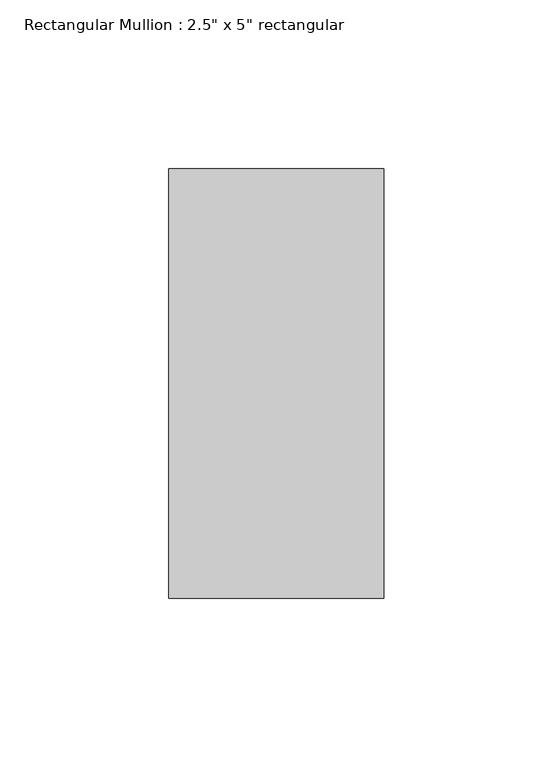
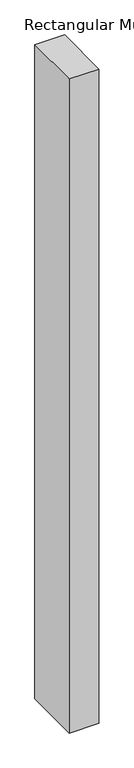
"""IFC4 building model written with IfcOpenShell, lengths in millimetres: member geometry."""

from ifc_helpers import new_model, si_unit, frame, origin, place, context, project, spatial, polyline, outline, extrude, source, transform, mapped, element, save


def member_921b0d60(model_context):
    return source(origin(), model_context, "Body", "SweptSolid", [
        extrude(outline(polyline([(0.0, 63.5), (0.0, -63.5), (-63.5, -63.5), (-63.5, 63.5), (0.0, 63.5)])), frame((0.0, 0.0, -1477.1971055), z_axis=(0.0, 0.0, 1.0), x_axis=(1.0, 0.0, 0.0)), (0.0, 0.0, 1.0), 1477.1971055),
    ])


if __name__ == "__main__":
    model = new_model("IFC4")
    model_context = context("Model", 3, world=origin())
    ifc_project = project(units=[si_unit("LENGTHUNIT", "METRE", prefix="MILLI")], contexts=[model_context])
    site = spatial("IfcSite", under=ifc_project)
    building = spatial("IfcBuilding", under=site)
    placement = place(None, origin())
    member_shape = member_921b0d60(model_context)
    element("IfcMember", 1, ObjectType="Rectangular Mullion : 2.5\" x 5\" rectangular", at=placement, inside=building, context=model_context, shape_type="MappedRepresentation", body=[
        mapped(member_shape, transform((0.0, 0.0, 0.0), x_axis=(1.0, 0.0, 0.0), y_axis=(0.0, 1.0, 0.0), z_axis=(0.0, 0.0, 1.0))),
    ])
    save(model, "model.ifc")

# Revit data of these elements
# Type "Rectangular Mullion : 2.5\" x 5\" rectangular"
#   built-in parameter 1007304 = 0.416667 (stored number, unit not read)
#   built-in parameter 1007301 = 0.104167 (stored number, unit not read)
#   built-in parameter 1007300 = 0.104167 (stored number, unit not read)
# Element 1 (IfcMember, "Rectangular Mullion : 2.5\" x 5\" rectangular")
#   Materials on its faces: "Aluminum"
# Materials
#   "Aluminum": class "Metal", colour RGB 247 247 247, transparency 0, Description = "Aluminum 6061", Cost = 0
